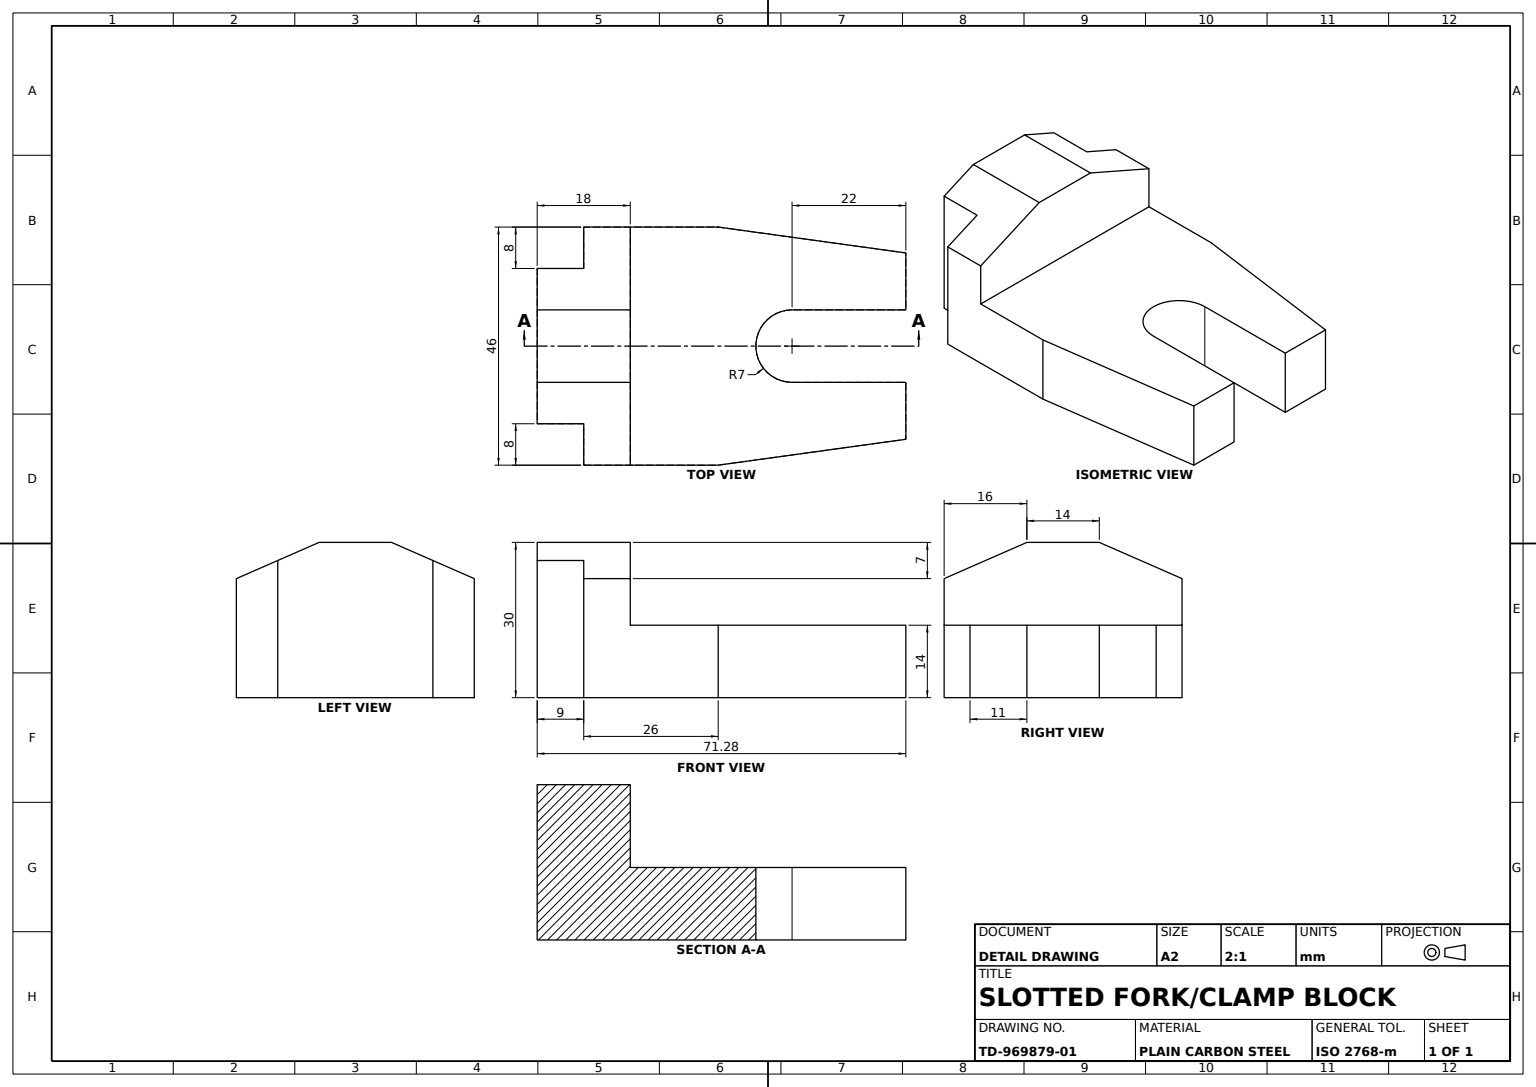
SolidWorks part; units mm, degrees
material "Plain Carbon Steel"
ref_plane "Front Plane" through (0, 0, 0) normal (0, 0, 1) x (1, 0, 0)
ref_plane "Top Plane" through (0, 0, 0) normal (0, 1, 0) x (1, 0, 0)
ref_plane "Right Plane" through (0, 0, 0) normal (1, 0, 0) x (0, 0, -1)
sketch "Base Plate Profile Sketch" plane through (0, 0, 0) normal (0, 1, 0) x (1, 0, 0)
  line L0 (0, 23) -> (0, -23)
  line L3 (62.2809, 7) -> (62.2809, 18)
  line L4 (62.2809, -7) -> (62.2809, -18)
  line L5 (0, 23) -> (26, 23)
  line L6 (0, -23) -> (26, -23)
  line L7 (26, 23) -> (62.2809, 18)
  line L8 (26, -23) -> (62.2809, -18)
  line L10 (40.2809, 7) -> (62.2809, 7)
  line L11 (40.2809, -7) -> (62.2809, -7)
  arc A0 (40.2809, 7) -> (40.2809, -7) centre (40.2809, 0) ccw
  point P4 (0, 0)
  point P10 (62.2809, 0)
  dimension "D7" = 14
  dimension "D1" = 46
  dimension "D2" = 14
  dimension "D3" = 11
  dimension "D4" = 11
  dimension "D5" = 26
  dimension "D6" = 22
  dimension "D8" = 62.2809
extrude "Base Plate 14mm with U-Slot" add sketch "Base Plate Profile Sketch" along normal mid plane 14
sketch "Raised Block Sketch" plane through (0, 0, 0) normal (-1, 0, 0) x (0, 0, 1)
  line L0 (-23, 7) -> (-23, 16)
  line L2 (-23, 7) -> (-23, -7)
  line L3 (-23, -7) -> (23, -7)
  line L4 (23, 7) -> (23, -7)
  line L5 (23, 7) -> (23, 16)
  line L7 (-7, 23) -> (7, 23)
  line L8 (-23, 16) -> (-7, 23)
  line L9 (7, 23) -> (23, 16)
  point P15 (0, 23)
  dimension "D1" = 9
  dimension "D2" = 9
  dimension "D3" = 23
  dimension "D4" = 14
extrude "Raised Block 18mm" add sketch "Raised Block Sketch" along normal mid plane 18
sketch "Step Cut Sketch" plane through (0, 23, 0) normal (0, 1, 0) x (1, 0, 0)
  line L1 (-9, 15) -> (0, 15)
  line L2 (0, 15) -> (0, 23)
  line L3 (-9, 23) -> (9, 23) construction
  line L4 (0, 23) -> (-9, 23)
  line L5 (-9, 23) -> (-9, 15)
  line L6 (-9, -23) -> (-9, -15)
  line L7 (0, -23) -> (-9, -23)
  line L8 (0, -15) -> (0, -23)
  line L9 (-9, -15) -> (0, -15)
  line L10 (-9, 7) -> (9, 7) construction
  point P3 (-9, 0)
  dimension "D1" = 8
  dimension "D2" = 7
  dimension "D3" = 22
extrude "Step Cut" cut sketch "Step Cut Sketch" against normal through all
